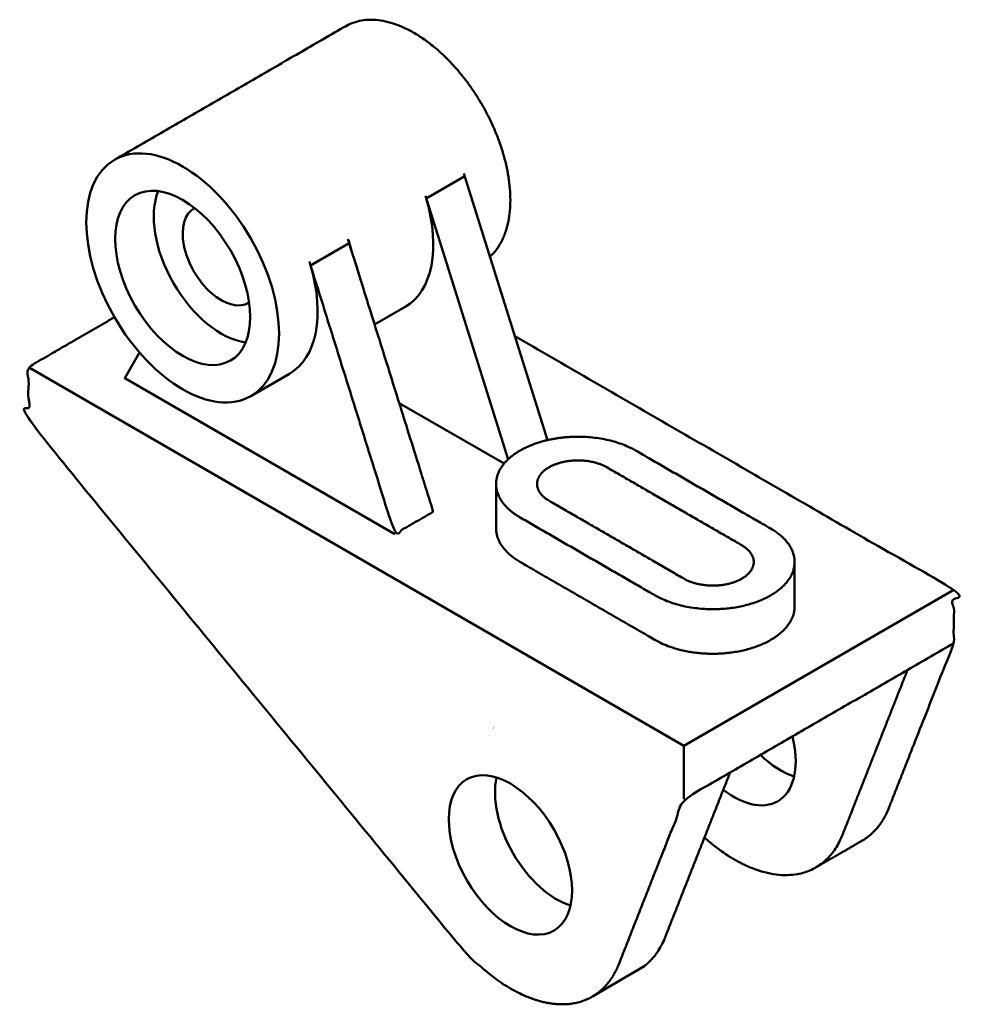
# Model space of a CAD drawing. Units: millimetres. Extents: x -24 to 189, y -68 to 153.
import ezdxf

# ---------------------------------------------------------------- set-up
doc = ezdxf.new("R2010")
doc.units = ezdxf.units.MM
doc.header["$MEASUREMENT"] = 0
doc.linetypes.add('CENTER', pattern=[2, 1.25, -0.25, 0.25, -0.25])
doc.layers.add('M-CONS', color=8, linetype='CENTER', lineweight=18)
doc.layers.add('M-OUTL', color=7, linetype='Continuous', lineweight=50)

msp = doc.modelspace()

# ---------------------------------------------------------------- linework, layer by layer
at = {"layer": 'M-CONS'}
for p, q in [((82.68, -5.49), (82.71, -5.5)), ((82.71, -5.5), (82.71, -5.5)), ((82.71, -5.5), (82.71, -5.5)), ((82.71, -5.5), (82.71, -5.5)), ((81.71, -7.23), (81.71, -7.23))]:
    msp.add_line(p, q, dxfattribs=at)
for points in [[(82.71, -5.5), (82.71, -5.5)], [(81.71, -7.23), (81.71, -7.23)]]:
    msp.add_lwpolyline(points, close=True, dxfattribs=at)
at = {"layer": 'M-OUTL'}
for p, q in [((67.57, 113.33), (76.23, 118.33)), ((94.82, 59.12), (76.06, 118.98)), ((85.97, 54.8), (67.44, 113.92)), ((41.59, 98.33), (50.25, 103.33)), ((55.98, 85.07), (62.82, 89.01)), ((-21.78, 75.53), (125.45, -9.47)), ((28.17, 69.01), (36.84, 74.01)), ((61.5, 67.45), (85.06, 53.85)), ((116.66, -58.85), (104.96, -65.75))]:
    msp.add_line(p, q, dxfattribs=at)
for points in [[(60.5, 38.03), (30.19, 55.53), (-0.12, 73.03), (3.18, 78.76)], [(186.07, 25.53), (125.45, -9.47), (125.45, -21.47)]]:
    msp.add_lwpolyline(points, dxfattribs=at)
for centre, major_axis in [((12.87, 95.53), (15.31, -26.52)), ((12.87, 95.53), (10.72, -18.56)), ((86.49, -33.98), (9.8, -16.97))]:
    msp.add_ellipse(centre, major_axis=major_axis, ratio=0.57735, dxfattribs=at)
for centre, major_axis, start_param, end_param in [((21.53, 100.53), (10.72, -18.56), 3.557545, 5.867233), ((47.51, 115.53), (15.31, -26.52), 0, 1.170274), ((21.53, 100.53), (6.12, -10.61), 3.119494, 6.305284), ((21.53, 100.53), (15.31, -26.52), 0, 1.170274), ((136.72, -4.98), (9.8, -16.97), 5.323021, 7.397083), ((147.12, 1.02), (9.8, -16.97), 5.169288, 5.724195), ((96.89, -27.98), (9.8, -16.97), 3.700583, 5.724195), ((136.72, -4.98), (18.37, -31.82), 4.991626, 5.001917)]:
    msp.add_ellipse(centre, major_axis=major_axis, ratio=0.57735, start_param=start_param, end_param=end_param, dxfattribs=at)
for points, weights, knots in [([(81.91, 100.31), (94.41, 111.64), (79.16, 135.99), (63.91, 160.35), (49.52, 152.05), (23.54, 137.05), (-2.44, 122.05)], [1, 0.728677607198, 1, 0.728677607198, 1, 1, 1], [0, 0, 0, 1.508815, 1.508815, 3.017629, 3.017629, 4.017629, 4.017629, 4.017629]), ([(50.92, 101.23), (50.58, 102.61), (50.13, 104.01), (50.08, 104.04), (50.03, 104.07), (59.59, 73.55), (69.16, 43.03), (64.83, 40.53), (60.5, 38.03), (50.91, 68.61), (41.33, 99.2)], [1, 0.998747497321, 1, 1, 1, 1, 1, 1, 1, 1, 1], [0, 0, 0, 0.100111, 0.100111, 1.100111, 1.100111, 2.100111, 2.100111, 3.100111, 3.100111, 4.100111, 4.100111, 4.100111]), ([(-2.44, 86.69), (-12.11, 81.11), (-21.78, 75.53), (-21.78, 69.53), (-21.78, 63.53), (26.06, 5.29), (73.9, -52.94), (84.33, -65.65), (95.52, -67.32), (106.7, -69), (110.85, -58.48), (118.15, -39.97), (125.45, -21.47), (155.76, -3.97), (186.07, 13.53)], [1, 1, 1, 1, 1, 1, 1, 0.908787454015, 1, 0.908787454015, 1, 1, 1, 1, 1], [0, 0, 0, 1, 1, 2, 2, 3, 3, 3.860855, 3.860855, 4.72171, 4.72171, 5.72171, 5.72171, 6.72171, 6.72171, 6.72171]), ([(155.09, -36.8), (160.29, -33.8), (165.49, -30.8), (169.5, -28.48), (171.47, -23.48), (178.77, -4.97), (186.07, 13.53), (186.07, 19.53), (186.07, 25.53), (136.79, 53.98), (87.51, 82.43)], [1, 1, 1, 0.976960326643, 1, 1, 1, 1, 1, 1, 1], [0, 0, 0, 1, 1, 1.430151, 1.430151, 2.430151, 2.430151, 3.430151, 3.430151, 4.430151, 4.430151, 4.430151]), ([(88.66, 41.77), (103.81, 33.02), (118.97, 24.27), (131.96, 16.77), (144.95, 24.27), (157.94, 31.77), (144.95, 39.27), (129.79, 48.02), (114.64, 56.77), (107.14, 61.1), (96.89, 59.52), (86.65, 57.93), (83.9, 52.02), (81.16, 46.1), (88.66, 41.77)], [1, 1, 1, 0.707106781187, 1, 0.707106781187, 1, 1, 1, 0.866025403784, 1, 0.866025403784, 1, 0.866025403784, 1], [0, 0, 0, 1, 1, 2.570796, 2.570796, 4.141593, 4.141593, 5.141593, 5.141593, 6.18879, 6.18879, 7.235988, 7.235988, 8.283185, 8.283185, 8.283185]), ([(108.14, 53.02), (104.39, 55.19), (99.27, 54.39), (94.15, 53.6), (92.78, 50.64), (91.4, 47.69), (95.15, 45.52), (102.73, 41.15), (110.31, 36.77), (117.89, 32.4), (125.46, 28.02), (129.21, 25.86), (134.34, 26.65), (139.46, 27.44), (140.83, 30.4), (142.2, 33.36), (138.45, 35.52), (130.88, 39.9), (123.3, 44.27), (115.72, 48.65), (108.14, 53.02)], [1, 0.866025403784, 1, 0.866025403784, 1, 0.866025403784, 1, 1, 1, 1, 1, 0.866025403784, 1, 0.866025403784, 1, 0.866025403784, 1, 1, 1, 1, 1], [0, 0, 0, 1.047198, 1.047198, 2.094395, 2.094395, 3.141593, 3.141593, 4.141593, 4.141593, 5.141593, 5.141593, 6.18879, 6.18879, 7.235988, 7.235988, 8.283185, 8.283185, 9.283185, 9.283185, 10.283185, 10.283185, 10.283185]), ([(83.28, 49.27), (83.28, 44.27), (83.28, 39.27), (83.28, 34.88), (88.66, 31.77), (103.81, 23.02), (118.97, 14.27), (127.65, 9.26), (138.99, 11.97), (150.33, 14.68), (150.33, 21.77), (150.33, 26.77), (150.33, 31.77)], [1, 1, 1, 0.923879532511, 1, 1, 1, 0.831469612303, 1, 0.831469612303, 1, 1, 1], [0, 0, 0, 1, 1, 1.785398, 1.785398, 2.785398, 2.785398, 3.963495, 3.963495, 5.141593, 5.141593, 6.141593, 6.141593, 6.141593]), ([(130.06, -30.13), (152.87, -50.29), (161.08, -29.48), (168.38, -10.97), (175.68, 7.53)], [1, 0.740180782695, 1, 1, 1], [0, 0, 0, 1.474914, 1.474914, 2.474914, 2.474914, 2.474914]), ([(113.93, -60.46), (118.94, -58.33), (121.24, -52.48), (128.54, -33.97), (135.84, -15.47)], [1, 0.968893705573, 1, 1, 1], [0, 0, 0, 0.500151, 0.500151, 1.500151, 1.500151, 1.500151])]:
    msp.add_rational_spline(points, weights, degree=2, knots=knots, dxfattribs=at)

doc.saveas('drawing.dxf')
